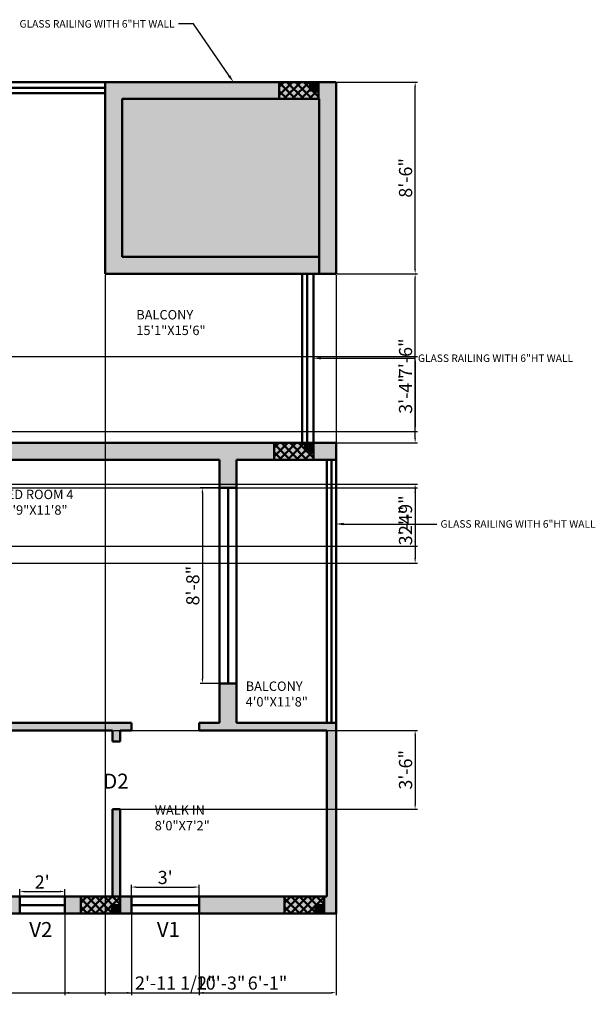
# Model space of a CAD drawing. Units: inches. Extents: x 1749 to 3550, y 1117 to 2383.
# Tile 15 of 15: x 3244 to 3550, y 1819 to 2343. Entities that reach past the tile are written whole.
import ezdxf
from ezdxf import colors
from ezdxf.entities.mleader import LeaderData, LeaderLine
from ezdxf.math import Vec2, Vec3

# ---------------------------------------------------------------- set-up
doc = ezdxf.new("R2010")
doc.units = ezdxf.units.IN
for name, color, linetype, lineweight in [('A-ANNO-DIMS', 2, 'Continuous', 18), ('A-ANNO-TEXT', 3, 'Continuous', 18), ('A-AREA-IDEN', 7, 'Continuous', 18), ('A-COLS', 10, 'Continuous', 50), ('A-WALL', 7, 'Continuous', 50), ('A-WALL-PATT', 8, 'Continuous', 13)]:
    doc.layers.add(name, color=color, linetype=linetype, lineweight=lineweight)
doc.styles.get("Standard").update_dxf_attribs({"font": 'arial.ttf'})
doc.dimstyles.new('ISO-25', dxfattribs={"dimtxt": 7, "dimasz": 2.5, "dimexe": 1.25, "dimexo": 0.625, "dimtad": 1, "dimdec": 1, "dimlunit": 3, "dimtxsty": 'Standard', "dimcen": 2.5, "dimadec": 0, "dimazin": 0, "dimtfac": 1, "dimtdec": 1, "dimtmove": 0, "dimatfit": 3, "dimfxl": 1, "dimarcsym": 0})

# ---------------------------------------------------------------- blocks, each defined once
blk = doc.blocks.new('*D134')
at = {"layer": 'A-ANNO-DIMS', "color": 0, "lineweight": -2, "ltscale": 0.5, "transparency": 16777216}
for p, q in [((3243.72, 1876.81), (3243.72, 1880.18)), ((3246.22, 1878.93), (3265.22, 1878.93)), ((3267.72, 1876.81), (3267.72, 1880.18))]:
    blk.add_line(p, q, dxfattribs=at)
at = {"layer": 'A-ANNO-DIMS', "color": 0, "ltscale": 0.5, "transparency": 16777216}
for points in [[(3246.22, 1879.35), (3246.22, 1878.51), (3243.72, 1878.93)], [(3265.22, 1879.35), (3265.22, 1878.51), (3267.72, 1878.93)]]:
    blk.add_solid(points, dxfattribs=at)
at = {"layer": 'Defpoints', "color": 0, "ltscale": 0.5, "transparency": 16777216}
for p in [(3243.72, 1876.18), (3267.72, 1878.93), (3267.72, 1876.18)]:
    blk.add_point(p, dxfattribs=at)
at = {"layer": 'A-ANNO-DIMS', "color": 0, "ltscale": 0.5, "transparency": 16777216, "insert": (3255.72, 1883.07), "char_height": 7, "attachment_point": 5}
blk.add_mtext("2'", dxfattribs=at)
blk = doc.blocks.new('*D135')
at = {"layer": 'A-ANNO-DIMS', "color": 0, "lineweight": -2, "ltscale": 0.5, "transparency": 16777216}
for p, q in [((3303.22, 1876.81), (3303.22, 1882.53)), ((3305.72, 1881.28), (3336.72, 1881.28)), ((3339.22, 1876.81), (3339.22, 1882.53))]:
    blk.add_line(p, q, dxfattribs=at)
at = {"layer": 'A-ANNO-DIMS', "color": 0, "ltscale": 0.5, "transparency": 16777216}
for points in [[(3305.72, 1881.69), (3305.72, 1880.86), (3303.22, 1881.28)], [(3336.72, 1881.69), (3336.72, 1880.86), (3339.22, 1881.28)]]:
    blk.add_solid(points, dxfattribs=at)
at = {"layer": 'Defpoints', "color": 0, "ltscale": 0.5, "transparency": 16777216}
for p in [(3339.22, 1881.28), (3303.22, 1876.18), (3339.22, 1876.18)]:
    blk.add_point(p, dxfattribs=at)
at = {"layer": 'A-ANNO-DIMS', "color": 0, "ltscale": 0.5, "transparency": 16777216, "insert": (3321.22, 1885.48), "char_height": 7, "attachment_point": 5}
blk.add_mtext("3'", dxfattribs=at)
blk = doc.blocks.new('*D136')
at = {"layer": 'A-ANNO-DIMS', "color": 0, "lineweight": -2, "ltscale": 0.5, "transparency": 16777216}
for p, q in [((3349.59, 2093.68), (3339.77, 2093.68)), ((3341.02, 2091.18), (3341.02, 1992.18)), ((3349.59, 1989.68), (3339.77, 1989.68))]:
    blk.add_line(p, q, dxfattribs=at)
at = {"layer": 'A-ANNO-DIMS', "color": 0, "ltscale": 0.5, "transparency": 16777216}
for points in [[(3340.6, 2091.18), (3341.43, 2091.18), (3341.02, 2093.68)], [(3340.6, 1992.18), (3341.43, 1992.18), (3341.02, 1989.68)]]:
    blk.add_solid(points, dxfattribs=at)
at = {"layer": 'Defpoints', "color": 0, "ltscale": 0.5, "transparency": 16777216}
for p in [(3350.22, 2093.68), (3341.02, 1989.68), (3350.22, 1989.68)]:
    blk.add_point(p, dxfattribs=at)
at = {"layer": 'A-ANNO-DIMS', "color": 0, "ltscale": 0.5, "transparency": 16777216, "insert": (3336.82, 2041.68), "char_height": 7, "attachment_point": 5, "rotation": 90}
blk.add_mtext('8\'-8"', dxfattribs=at)
blk = doc.blocks.new('*D180')
at = {"layer": 'A-ANNO-DIMS', "color": 0, "lineweight": -2, "ltscale": 0.5, "transparency": 16777216}
for p, q in [((2745.22, 1866.56), (2745.22, 1823.83)), ((3412.22, 1866.56), (3412.22, 1823.83)), ((2747.72, 1825.08), (3409.72, 1825.08))]:
    blk.add_line(p, q, dxfattribs=at)
at = {"layer": 'A-ANNO-DIMS', "color": 0, "ltscale": 0.5, "transparency": 16777216}
for points in [[(2747.72, 1825.5), (2747.72, 1824.66), (2745.22, 1825.08)], [(3409.72, 1825.5), (3409.72, 1824.66), (3412.22, 1825.08)]]:
    blk.add_solid(points, dxfattribs=at)
at = {"layer": 'Defpoints', "color": 0, "ltscale": 0.5, "transparency": 16777216}
for p in [(2745.22, 1867.18), (3412.22, 1867.18), (3412.22, 1825.08)]:
    blk.add_point(p, dxfattribs=at)
at = {"layer": 'A-ANNO-DIMS', "color": 0, "ltscale": 0.5, "transparency": 16777216, "insert": (3078.72, 1829.27), "char_height": 7, "attachment_point": 5}
blk.add_mtext('55\'-7"', dxfattribs=at)
blk = doc.blocks.new('*D183')
at = {"layer": 'A-ANNO-DIMS', "color": 0, "lineweight": -2, "ltscale": 0.5, "transparency": 16777216}
for p, q in [((3289.22, 2207.06), (3289.22, 1823.83)), ((3412.22, 2207.06), (3412.22, 1823.83)), ((3291.72, 1825.08), (3409.72, 1825.08))]:
    blk.add_line(p, q, dxfattribs=at)
at = {"layer": 'A-ANNO-DIMS', "color": 0, "ltscale": 0.5, "transparency": 16777216}
for points in [[(3291.72, 1825.5), (3291.72, 1824.66), (3289.22, 1825.08)], [(3409.72, 1825.5), (3409.72, 1824.66), (3412.22, 1825.08)]]:
    blk.add_solid(points, dxfattribs=at)
at = {"layer": 'Defpoints', "color": 0, "ltscale": 0.5, "transparency": 16777216}
for p in [(3289.22, 2207.68), (3412.22, 2207.68), (3412.22, 1825.08)]:
    blk.add_point(p, dxfattribs=at)
at = {"layer": 'A-ANNO-DIMS', "color": 0, "ltscale": 0.5, "transparency": 16777216, "insert": (3350.72, 1829.28), "char_height": 7, "attachment_point": 5}
blk.add_mtext('10\'-3"', dxfattribs=at)
blk = doc.blocks.new('*D187')
at = {"layer": 'A-ANNO-DIMS', "color": 0, "lineweight": -2, "ltscale": 0.5, "transparency": 16777216}
for p, q in [((3267.72, 1866.56), (3267.72, 1823.83)), ((3303.22, 1866.56), (3303.22, 1823.83)), ((3270.22, 1825.08), (3300.72, 1825.08)), ((3303.22, 1825.08), (3347.45, 1825.08))]:
    blk.add_line(p, q, dxfattribs=at)
at = {"layer": 'A-ANNO-DIMS', "color": 0, "ltscale": 0.5, "transparency": 16777216}
for points in [[(3270.22, 1825.5), (3270.22, 1824.66), (3267.72, 1825.08)], [(3300.72, 1825.5), (3300.72, 1824.66), (3303.22, 1825.08)]]:
    blk.add_solid(points, dxfattribs=at)
at = {"layer": 'Defpoints', "color": 0, "ltscale": 0.5, "transparency": 16777216}
for p in [(3267.72, 1867.18), (3303.22, 1867.18), (3303.22, 1825.08)]:
    blk.add_point(p, dxfattribs=at)
at = {"layer": 'A-ANNO-DIMS', "color": 0, "ltscale": 0.5, "transparency": 16777216, "insert": (3326.58, 1829.33), "char_height": 7, "attachment_point": 5}
blk.add_mtext('2\'-11 1/2"', dxfattribs=at)
blk = doc.blocks.new('*D188')
at = {"layer": 'A-ANNO-DIMS', "color": 0, "lineweight": -2, "ltscale": 0.5, "transparency": 16777216}
for p, q in [((3339.22, 1866.56), (3339.22, 1823.83)), ((3412.22, 1866.56), (3412.22, 1823.83)), ((3341.72, 1825.08), (3409.72, 1825.08))]:
    blk.add_line(p, q, dxfattribs=at)
at = {"layer": 'A-ANNO-DIMS', "color": 0, "ltscale": 0.5, "transparency": 16777216}
for points in [[(3341.72, 1825.5), (3341.72, 1824.66), (3339.22, 1825.08)], [(3409.72, 1825.5), (3409.72, 1824.66), (3412.22, 1825.08)]]:
    blk.add_solid(points, dxfattribs=at)
at = {"layer": 'Defpoints', "color": 0, "ltscale": 0.5, "transparency": 16777216}
for p in [(3339.22, 1867.18), (3412.22, 1867.18), (3412.22, 1825.08)]:
    blk.add_point(p, dxfattribs=at)
at = {"layer": 'A-ANNO-DIMS', "color": 0, "ltscale": 0.5, "transparency": 16777216, "insert": (3375.72, 1829.28), "char_height": 7, "attachment_point": 5}
blk.add_mtext('6\'-1"', dxfattribs=at)
blk = doc.blocks.new('*D189')
at = {"layer": 'A-ANNO-DIMS', "color": 0, "lineweight": -2, "ltscale": 0.5, "transparency": 16777216}
for p, q in [((3412.84, 2207.68), (3455.57, 2207.68)), ((3454.32, 2120.18), (3454.32, 2205.18)), ((3412.84, 2117.68), (3455.57, 2117.68))]:
    blk.add_line(p, q, dxfattribs=at)
at = {"layer": 'A-ANNO-DIMS', "color": 0, "ltscale": 0.5, "transparency": 16777216}
for points in [[(3453.9, 2205.18), (3454.74, 2205.18), (3454.32, 2207.68)], [(3453.9, 2120.18), (3454.74, 2120.18), (3454.32, 2117.68)]]:
    blk.add_solid(points, dxfattribs=at)
at = {"layer": 'Defpoints', "color": 0, "ltscale": 0.5, "transparency": 16777216}
for p in [(3412.22, 2207.68), (3454.32, 2207.68), (3412.22, 2117.68)]:
    blk.add_point(p, dxfattribs=at)
at = {"layer": 'A-ANNO-DIMS', "color": 0, "ltscale": 0.5, "transparency": 16777216, "insert": (3450.12, 2162.68), "char_height": 7, "attachment_point": 5, "rotation": 90}
blk.add_mtext('7\'-6"', dxfattribs=at)
blk = doc.blocks.new('*D190')
at = {"layer": 'A-ANNO-DIMS', "color": 0, "lineweight": -2, "ltscale": 0.5, "transparency": 16777216}
for p, q in [((3412.84, 2309.68), (3455.57, 2309.68)), ((3454.32, 2210.18), (3454.32, 2307.18)), ((3412.84, 2207.68), (3455.57, 2207.68))]:
    blk.add_line(p, q, dxfattribs=at)
at = {"layer": 'A-ANNO-DIMS', "color": 0, "ltscale": 0.5, "transparency": 16777216}
for points in [[(3453.9, 2307.18), (3454.74, 2307.18), (3454.32, 2309.68)], [(3453.9, 2210.18), (3454.74, 2210.18), (3454.32, 2207.68)]]:
    blk.add_solid(points, dxfattribs=at)
at = {"layer": 'Defpoints', "color": 0, "ltscale": 0.5, "transparency": 16777216}
for p in [(3412.22, 2309.68), (3454.32, 2309.68), (3412.22, 2207.68)]:
    blk.add_point(p, dxfattribs=at)
at = {"layer": 'A-ANNO-DIMS', "color": 0, "ltscale": 0.5, "transparency": 16777216, "insert": (3450.12, 2258.68), "char_height": 7, "attachment_point": 5, "rotation": 90}
blk.add_mtext('8\'-6"', dxfattribs=at)
blk = doc.blocks.new('*D191')
at = {"layer": 'A-ANNO-DIMS', "color": 0, "lineweight": -2, "ltscale": 0.5, "transparency": 16777216}
for p, q in [((2998.84, 2163.68), (3455.57, 2163.68)), ((3454.32, 2161.18), (3454.32, 2126.18)), ((2998.84, 2123.68), (3455.57, 2123.68))]:
    blk.add_line(p, q, dxfattribs=at)
at = {"layer": 'A-ANNO-DIMS', "color": 0, "ltscale": 0.5, "transparency": 16777216}
for points in [[(3453.9, 2161.18), (3454.74, 2161.18), (3454.32, 2163.68)], [(3453.9, 2126.18), (3454.74, 2126.18), (3454.32, 2123.68)]]:
    blk.add_solid(points, dxfattribs=at)
at = {"layer": 'Defpoints', "color": 0, "ltscale": 0.5, "transparency": 16777216}
for p in [(2998.22, 2163.68), (2998.22, 2123.68), (3454.32, 2123.68)]:
    blk.add_point(p, dxfattribs=at)
at = {"layer": 'A-ANNO-DIMS', "color": 0, "ltscale": 0.5, "transparency": 16777216, "insert": (3450.12, 2143.68), "char_height": 7, "attachment_point": 5, "rotation": 90}
blk.add_mtext('3\'-4"', dxfattribs=at)
blk = doc.blocks.new('*D193')
at = {"layer": 'A-ANNO-DIMS', "color": 0, "lineweight": -2, "ltscale": 0.5, "transparency": 16777216}
for p, q in [((3169.84, 2093.68), (3455.57, 2093.68)), ((3454.32, 2091.18), (3454.32, 2056.18)), ((3169.84, 2053.68), (3455.57, 2053.68))]:
    blk.add_line(p, q, dxfattribs=at)
at = {"layer": 'A-ANNO-DIMS', "color": 0, "ltscale": 0.5, "transparency": 16777216}
for points in [[(3453.9, 2091.18), (3454.74, 2091.18), (3454.32, 2093.68)], [(3453.9, 2056.18), (3454.74, 2056.18), (3454.32, 2053.68)]]:
    blk.add_solid(points, dxfattribs=at)
at = {"layer": 'Defpoints', "color": 0, "ltscale": 0.5, "transparency": 16777216}
for p in [(3169.22, 2093.68), (3169.22, 2053.68), (3454.32, 2053.68)]:
    blk.add_point(p, dxfattribs=at)
at = {"layer": 'A-ANNO-DIMS', "color": 0, "ltscale": 0.5, "transparency": 16777216, "insert": (3450.12, 2073.68), "char_height": 7, "attachment_point": 5, "rotation": 90}
blk.add_mtext('3\'-4"', dxfattribs=at)
blk = doc.blocks.new('*D196')
at = {"layer": 'A-ANNO-DIMS', "color": 0, "lineweight": -2, "ltscale": 0.5, "transparency": 16777216}
for p, q in [((3293.84, 1964.68), (3455.57, 1964.68)), ((3454.32, 1962.18), (3454.32, 1925.18)), ((3293.84, 1922.68), (3455.57, 1922.68))]:
    blk.add_line(p, q, dxfattribs=at)
at = {"layer": 'A-ANNO-DIMS', "color": 0, "ltscale": 0.5, "transparency": 16777216}
for points in [[(3453.9, 1962.18), (3454.74, 1962.18), (3454.32, 1964.68)], [(3453.9, 1925.18), (3454.74, 1925.18), (3454.32, 1922.68)]]:
    blk.add_solid(points, dxfattribs=at)
at = {"layer": 'Defpoints', "color": 0, "ltscale": 0.5, "transparency": 16777216}
for p in [(3293.22, 1964.68), (3293.22, 1922.68), (3454.32, 1922.68)]:
    blk.add_point(p, dxfattribs=at)
at = {"layer": 'A-ANNO-DIMS', "color": 0, "ltscale": 0.5, "transparency": 16777216, "insert": (3450.12, 1943.68), "char_height": 7, "attachment_point": 5, "rotation": 90}
blk.add_mtext('3\'-6"', dxfattribs=at)
blk = doc.blocks.new('*D197')
at = {"layer": 'A-ANNO-DIMS', "color": 0, "lineweight": -2, "ltscale": 0.5, "transparency": 16777216}
for p, q in [((2823.84, 2095.68), (3455.57, 2095.68)), ((3454.32, 2093.18), (3454.32, 2065.18)), ((2823.84, 2062.68), (3455.57, 2062.68))]:
    blk.add_line(p, q, dxfattribs=at)
at = {"layer": 'A-ANNO-DIMS', "color": 0, "ltscale": 0.5, "transparency": 16777216}
for points in [[(3453.9, 2093.18), (3454.74, 2093.18), (3454.32, 2095.68)], [(3453.9, 2065.18), (3454.74, 2065.18), (3454.32, 2062.68)]]:
    blk.add_solid(points, dxfattribs=at)
at = {"layer": 'Defpoints', "color": 0, "ltscale": 0.5, "transparency": 16777216}
for p in [(2823.22, 2095.68), (2823.22, 2062.68), (3454.32, 2062.68)]:
    blk.add_point(p, dxfattribs=at)
at = {"layer": 'A-ANNO-DIMS', "color": 0, "ltscale": 0.5, "transparency": 16777216, "insert": (3450.12, 2079.18), "char_height": 7, "attachment_point": 5, "rotation": 90}
blk.add_mtext('2\'-9"', dxfattribs=at)

msp = doc.modelspace()

# ---------------------------------------------------------------- hatches: boundary and pattern name
at = {"layer": 'A-COLS', "ltscale": 10}
h = msp.add_hatch(dxfattribs=at)
h.set_pattern_fill('ANSI37', color=256, angle=360)
h.set_pattern_definition([(45, (1730.631, 965.6985), (-2.245064, 2.245064), []), (135, (1730.631, 965.6985), (-2.245064, -2.245064), [])])
h.paths.add_polyline_path([(3381.88, 2309.68), (3381.88, 2300.68), (3402.88, 2300.68), (3402.88, 2309.68)])
h = msp.add_hatch(color=256, dxfattribs=at)
h.dxf.hatch_style = 1
h.paths.add_polyline_path([(3402.88, 2309.68), (3398.38, 2309.68), (3398.38, 2305.18), (3402.88, 2305.18)])
h = msp.add_hatch(dxfattribs=at)
h.set_pattern_fill('ANSI37', color=256, angle=360)
h.set_pattern_definition([(45, (1727.9752, 728.6265), (-2.245064, 2.245064), []), (135, (1727.9752, 728.6265), (-2.245064, -2.245064), [])])
h.paths.add_polyline_path([(3379.22, 2117.68), (3379.22, 2108.68), (3400.22, 2108.68), (3400.22, 2117.68)])
h = msp.add_hatch(color=256, dxfattribs=at)
h.dxf.hatch_style = 1
h.paths.add_polyline_path([(3400.22, 2117.68), (3395.72, 2117.68), (3395.72, 2113.18), (3400.22, 2113.18)])
h = msp.add_hatch(dxfattribs=at)
h.set_pattern_fill('ANSI37', color=256, angle=360)
h.set_pattern_definition([(45, (1624.9752, 509.075), (-2.245064, 2.245064), []), (135, (1624.9752, 509.075), (-2.245064, -2.245064), [])])
h.paths.add_polyline_path([(3297.22, 1867.18), (3297.22, 1876.18), (3276.22, 1876.18), (3276.22, 1867.18)])
h = msp.add_hatch(dxfattribs=at)
h.set_pattern_fill('ANSI37', color=256, angle=360)
h.set_pattern_definition([(45, (1733.5644, 509.075), (-2.245064, 2.245064), []), (135, (1733.5644, 509.075), (-2.245064, -2.245064), [])])
h.paths.add_polyline_path([(3405.81, 1867.18), (3405.81, 1876.18), (3384.81, 1876.18), (3384.81, 1867.18)])
h = msp.add_hatch(color=256, dxfattribs=at)
h.dxf.hatch_style = 1
h.paths.add_polyline_path([(3297.22, 1871.68), (3292.72, 1871.68), (3292.72, 1867.18), (3297.22, 1867.18)])
h = msp.add_hatch(color=256, dxfattribs=at)
h.dxf.hatch_style = 1
h.paths.add_polyline_path([(3405.81, 1871.68), (3401.31, 1871.68), (3401.31, 1867.18), (3405.81, 1867.18)])
at = {"layer": 'A-WALL-PATT', "ltscale": 0.5}
h = msp.add_hatch(color=256, dxfattribs=at)
h.dxf.hatch_style = 1
h.paths.add_polyline_path([(3289.22, 2207.68), (3403.22, 2207.68), (3403.22, 2216.68), (3298.22, 2216.68), (3298.22, 2300.68), (3403.22, 2300.68), (3403.22, 2207.68), (3412.22, 2207.68), (3412.22, 2309.68), (3289.22, 2309.68)])
h = msp.add_hatch(color=256, dxfattribs=at)
h.dxf.hatch_style = 1
h.paths.add_polyline_path([(3298.22, 2216.68), (3403.22, 2216.68), (3403.22, 2300.68), (3298.22, 2300.68)])
h = msp.add_hatch(color=256, dxfattribs=at)
h.dxf.hatch_style = 1
h.paths.add_polyline_path([(3289.22, 2108.68), (3350.22, 2108.68), (3350.22, 2093.68), (3359.22, 2093.68), (3359.22, 2108.68), (3412.22, 2108.68), (3412.22, 2117.68), (3289.22, 2117.68), (3178.22, 2117.68), (3169.22, 2117.68), (3169.22, 2093.68), (3173.22, 2093.68), (3173.22, 2108.68)])
h = msp.add_hatch(color=256, dxfattribs=at)
h.dxf.hatch_style = 1
h.paths.add_polyline_path([(3303.22, 1968.68), (3289.22, 1968.68), (3173.22, 1968.68), (3173.22, 2053.68), (3169.22, 2053.68), (3169.22, 1964.68), (3169.22, 1890.68), (3163.22, 1890.68), (3163.22, 1881.68), (3169.22, 1881.68), (3169.22, 1867.18), (3243.72, 1867.18), (3243.72, 1876.18), (3173.22, 1876.18), (3173.22, 1964.68), (3289.22, 1964.68), (3293.22, 1964.68), (3293.22, 1958.68), (3297.22, 1958.68), (3297.22, 1964.68), (3303.22, 1964.68)])
h = msp.add_hatch(color=256, dxfattribs=at)
h.dxf.hatch_style = 1
h.paths.add_polyline_path([(3350.22, 1968.68), (3339.22, 1968.68), (3339.22, 1964.68), (3407.22, 1964.68), (3407.22, 1876.18), (3339.22, 1876.18), (3339.22, 1867.18), (3412.22, 1867.18), (3412.22, 1968.68), (3359.22, 1968.68), (3359.22, 1989.68), (3350.22, 1989.68)])
h = msp.add_hatch(color=256, dxfattribs=at)
h.dxf.hatch_style = 1
h.paths.add_polyline_path([(3297.22, 1922.68), (3293.22, 1922.68), (3293.22, 1876.18), (3267.72, 1876.18), (3267.72, 1867.18), (3303.22, 1867.18), (3303.22, 1876.18), (3297.22, 1876.18)])

# ---------------------------------------------------------------- linework, layer by layer
at = {"layer": 'A-COLS', "ltscale": 10}
for points in [[(3381.88, 2300.68), (3402.88, 2300.68), (3402.88, 2309.68), (3381.88, 2309.68)], [(3402.88, 2305.18), (3402.88, 2309.68), (3398.38, 2309.68), (3398.38, 2305.18)], [(3379.22, 2108.68), (3400.22, 2108.68), (3400.22, 2117.68), (3379.22, 2117.68)], [(3400.22, 2113.18), (3400.22, 2117.68), (3395.72, 2117.68), (3395.72, 2113.18)], [(3276.22, 1876.18), (3297.22, 1876.18), (3297.22, 1867.18), (3276.22, 1867.18)], [(3384.81, 1876.18), (3405.81, 1876.18), (3405.81, 1867.18), (3384.81, 1867.18)], [(3297.22, 1871.68), (3297.22, 1867.18), (3292.72, 1867.18), (3292.72, 1871.68)], [(3405.81, 1871.68), (3405.81, 1867.18), (3401.31, 1867.18), (3401.31, 1871.68)]]:
    msp.add_lwpolyline(points, close=True, dxfattribs=at)
at = {"layer": 'A-WALL', "ltscale": 0.5}
for p, q in [((2745.22, 2309.68), (3412.22, 2309.68)), ((3178.22, 2306.68), (3289.22, 2306.68)), ((3289.22, 2309.68), (3289.22, 2207.68)), ((3412.22, 2309.68), (3412.22, 2207.68)), ((3178.22, 2303.68), (3289.22, 2303.68)), ((3298.22, 2300.68), (3298.22, 2216.68)), ((3298.22, 2300.68), (3403.22, 2300.68)), ((3403.22, 2300.68), (3403.22, 2207.68)), ((3298.22, 2216.68), (3403.22, 2216.68)), ((3289.22, 2207.68), (3412.22, 2207.68)), ((3394.22, 2207.68), (3394.22, 2117.68)), ((3396.9, 2117.68), (3396.9, 2207.68)), ((3400.22, 2207.68), (3400.22, 2117.68)), ((3178.22, 2117.68), (3289.22, 2117.68)), ((3289.22, 2117.68), (3412.22, 2117.68)), ((3412.22, 2117.68), (3412.22, 2108.68)), ((3173.22, 2108.68), (3289.22, 2108.68)), ((3289.22, 2108.68), (3350.22, 2108.68)), ((3350.22, 2108.68), (3350.22, 1968.68)), ((3359.22, 2108.68), (3359.22, 1968.68)), ((3359.22, 2108.68), (3412.22, 2108.68)), ((3407.22, 2108.68), (3407.22, 1968.68)), ((3409.77, 2108.68), (3409.77, 1968.68)), ((3412.22, 2108.68), (3412.22, 1867.18)), ((3359.22, 2093.68), (3350.22, 2093.68)), ((3354.72, 2093.68), (3354.72, 1989.68)), ((3359.22, 1989.68), (3350.22, 1989.68)), ((3173.22, 1968.68), (3289.22, 1968.68)), ((3289.22, 1968.68), (3303.22, 1968.68)), ((3303.22, 1964.68), (3303.22, 1968.68)), ((3339.22, 1964.68), (3339.22, 1968.68)), ((3339.22, 1968.68), (3350.22, 1968.68)), ((3359.22, 1968.68), (3412.22, 1968.68)), ((3173.22, 1964.68), (3289.22, 1964.68)), ((3289.22, 1964.68), (3293.22, 1964.68)), ((3293.22, 1964.68), (3293.22, 1958.68)), ((3297.22, 1964.68), (3297.22, 1958.68)), ((3297.22, 1964.68), (3303.22, 1964.68)), ((3339.22, 1964.68), (3407.22, 1964.68)), ((3407.22, 1964.68), (3407.22, 1876.18)), ((3297.22, 1958.68), (3293.22, 1958.68)), ((3297.22, 1922.68), (3293.22, 1922.68)), ((3293.22, 1922.68), (3293.22, 1876.18)), ((3297.22, 1922.68), (3297.22, 1876.18)), ((3173.22, 1876.18), (3293.22, 1876.18)), ((3243.72, 1876.18), (3243.72, 1867.18)), ((3267.72, 1876.18), (3267.72, 1867.18)), ((3297.22, 1876.18), (3407.22, 1876.18)), ((3303.22, 1876.18), (3303.22, 1867.18)), ((3339.22, 1876.18), (3339.22, 1867.18)), ((3243.72, 1871.68), (3267.72, 1871.68)), ((3303.22, 1871.68), (3339.22, 1871.68)), ((3169.22, 1867.18), (3412.22, 1867.18))]:
    msp.add_line(p, q, dxfattribs=at)

# ---------------------------------------------------------------- texts
at = {"layer": 'A-ANNO-TEXT', "ltscale": 0.5}
for s, p in [('D2', (3288.18, 1933.64)), ('V2', (3248.81, 1854.66)), ('V1', (3316.77, 1854.77))]:
    msp.add_text(s, height=8, dxfattribs=at).set_placement(p)
at = {"layer": 'A-AREA-IDEN', "ltscale": 0.5}
for s, p in [('BALCONY', (3305.83, 2183.34)), ('15\'1"X15\'6"', (3305.83, 2175.04)), ('BED ROOM 4', (3232.33, 2087.73)), ('14\'9"X11\'8"', (3232.33, 2079.43)), ('BALCONY', (3364.09, 1985.68)), ('4\'0"X11\'8"', (3364.09, 1977.38)), ('WALK IN', (3315.63, 1919.77)), ('8\'0"X7\'2"', (3315.63, 1911.47))]:
    msp.add_text(s, height=5, dxfattribs=at).set_placement(p)

# ---------------------------------------------------------------- dimensions: what is measured, and where the dimension line sits
at = {"layer": 'A-ANNO-DIMS', "ltscale": 0.5}
for base, p1, p2, override, picture, middle in [((3454.32, 2309.68), (3412.22, 2207.68), (3412.22, 2309.68), {"dimdec": 1, "dimlfac": 1, "dimrnd": 0, "dimzin": 1, "dimdsep": 46, "dimlunit": 4, "dimfrac": 2}, '*D190', (3450.12, 2258.68)), ((3454.32, 2207.68), (3412.22, 2117.68), (3412.22, 2207.68), {"dimdec": 1, "dimlfac": 1, "dimrnd": 0, "dimzin": 1, "dimdsep": 46, "dimlunit": 4, "dimfrac": 2}, '*D189', (3450.12, 2162.68)), ((3454.32, 2123.68), (2998.22, 2163.68), (2998.22, 2123.68), {"dimdec": 1, "dimlfac": 1, "dimrnd": 0, "dimzin": 1, "dimdsep": 46, "dimlunit": 4, "dimfrac": 2}, '*D191', (3450.12, 2143.68)), ((3454.32, 2062.68), (2823.22, 2095.68), (2823.22, 2062.68), {"dimdec": 1, "dimlfac": 1, "dimrnd": 0, "dimzin": 1, "dimdsep": 46, "dimlunit": 4, "dimfrac": 2}, '*D197', (3450.12, 2079.18)), ((3454.32, 2053.68), (3169.22, 2093.68), (3169.22, 2053.68), {"dimdec": 1, "dimlfac": 1, "dimrnd": 0, "dimzin": 1, "dimdsep": 46, "dimlunit": 4, "dimfrac": 2}, '*D193', (3450.12, 2073.68)), ((3341.02, 1989.68), (3350.22, 2093.68), (3350.22, 1989.68), {"dimclrd": 0, "dimclre": 0, "dimclrt": 0}, '*D136', (3336.82, 2041.68)), ((3454.32, 1922.68), (3293.22, 1964.68), (3293.22, 1922.68), {"dimdec": 1, "dimlfac": 1, "dimrnd": 0, "dimzin": 1, "dimdsep": 46, "dimlunit": 4, "dimfrac": 2}, '*D196', (3450.12, 1943.68))]:
    dim = msp.add_linear_dim(base=base, p1=p1, p2=p2, angle=90, dimstyle='ISO-25', override=override, dxfattribs=at)
    dim.commit()
    dim.dimension.update_dxf_attribs({"geometry": picture, "text_midpoint": middle})
for base, p1, p2, override, picture, middle in [((3412.22, 1825.08), (3289.22, 2207.68), (3412.22, 2207.68), {"dimdec": 1, "dimlfac": 1, "dimrnd": 0, "dimzin": 1, "dimdsep": 46, "dimlunit": 4, "dimfrac": 2}, '*D183', (3350.72, 1829.28)), ((3267.72, 1878.93), (3243.72, 1876.18), (3267.72, 1876.18), {"dimclrd": 0, "dimclre": 0, "dimclrt": 0}, '*D134', (3255.72, 1883.07)), ((3339.22, 1881.28), (3303.22, 1876.18), (3339.22, 1876.18), {"dimclrd": 0, "dimclre": 0, "dimclrt": 0}, '*D135', (3321.22, 1885.48)), ((3412.22, 1825.08), (2745.22, 1867.18), (3412.22, 1867.18), {"dimdec": 1, "dimlfac": 1, "dimrnd": 0, "dimzin": 1, "dimdsep": 46, "dimlunit": 4, "dimfrac": 2}, '*D180', (3078.72, 1829.27)), ((3303.22, 1825.08), (3267.72, 1867.18), (3303.22, 1867.18), {"dimdec": 1, "dimlfac": 1, "dimrnd": 0, "dimzin": 1, "dimdsep": 46, "dimlunit": 4, "dimfrac": 2}, '*D187', (3326.58, 1829.33)), ((3412.22, 1825.08), (3339.22, 1867.18), (3412.22, 1867.18), {"dimdec": 1, "dimlfac": 1, "dimrnd": 0, "dimzin": 1, "dimdsep": 46, "dimlunit": 4, "dimfrac": 2}, '*D188', (3375.72, 1829.28))]:
    dim = msp.add_linear_dim(base=base, p1=p1, p2=p2, dimstyle='ISO-25', override=override, dxfattribs=at)
    dim.commit()
    dim.dimension.update_dxf_attribs({"geometry": picture, "text_midpoint": middle})

# ---------------------------------------------------------------- leaders
at = {"layer": 'A-ANNO-TEXT', "ltscale": 0.5}
ml = msp.add_multileader_mtext('Standard', dxfattribs=at)
ml.set_content('GLASS RAILING WITH 6"HT WALL', color=256)
ml.set_leader_properties()
ml.build(insert=Vec2(0, 0))
ctx = ml.context
ctx.base_point, ctx.plane_origin = Vec3(3235.5, 2340.62), Vec3(3357.56, 2309.68)
ctx.text_align_type = 2
notes = []
notes.append((ctx, [(0, (1, 1, 0), (3336.24, 2340.62), (-1, 0), 8, [(0, [(3357.56, 2309.68)], 0, [])])]))
ctx.mtext.insert, ctx.mtext.alignment, ctx.mtext.flow_direction = Vec3(3326.24, 2342.66), 3, 5
ml = msp.add_multileader_mtext('Standard', dxfattribs=at)
ml.set_content('GLASS RAILING WITH 6"HT WALL', color=256)
ml.set_leader_properties()
ml.build(insert=Vec2(0, 0))
ctx = ml.context
ctx.base_point, ctx.plane_origin = Vec3(3453.82, 2162.68), Vec3(3400.22, 2162.68)
notes.append((ctx, [(0, (1, 1, 0), (3445.82, 2162.68), (1, 0), 8, [(0, [(3400.22, 2162.68)], 0, [])])]))
ctx.mtext.insert, ctx.mtext.flow_direction = Vec3(3455.82, 2164.72), 5
ml = msp.add_multileader_mtext('Standard', dxfattribs=at)
ml.set_content('GLASS RAILING WITH 6"HT WALL', color=256)
ml.set_leader_properties()
ml.build(insert=Vec2(0, 0))
ctx = ml.context
ctx.base_point, ctx.plane_origin = Vec3(3465.82, 2074.49), Vec3(3412.22, 2074.49)
notes.append((ctx, [(0, (1, 1, 0), (3457.82, 2074.49), (1, 0), 8, [(0, [(3412.22, 2074.49)], 0, [])])]))
ctx.mtext.insert, ctx.mtext.flow_direction = Vec3(3467.82, 2076.52), 5
for ctx, leaders in notes:
    for number, flags, end, landing, length, lines in leaders:
        leader = LeaderData()
        leader.index, (leader.has_last_leader_line, leader.has_dogleg_vector, leader.attachment_direction) = number, flags
        leader.last_leader_point, leader.dogleg_vector, leader.dogleg_length = Vec3(end), Vec3(landing), length
        for number, points, colour, breaks in lines:
            line = LeaderLine()
            line.index, line.vertices, line.color, line.breaks = number, Vec3.list(points), colors.encode_raw_color(colour), breaks
            leader.lines.append(line)
        ctx.leaders.append(leader)

doc.saveas('drawing.dxf')
